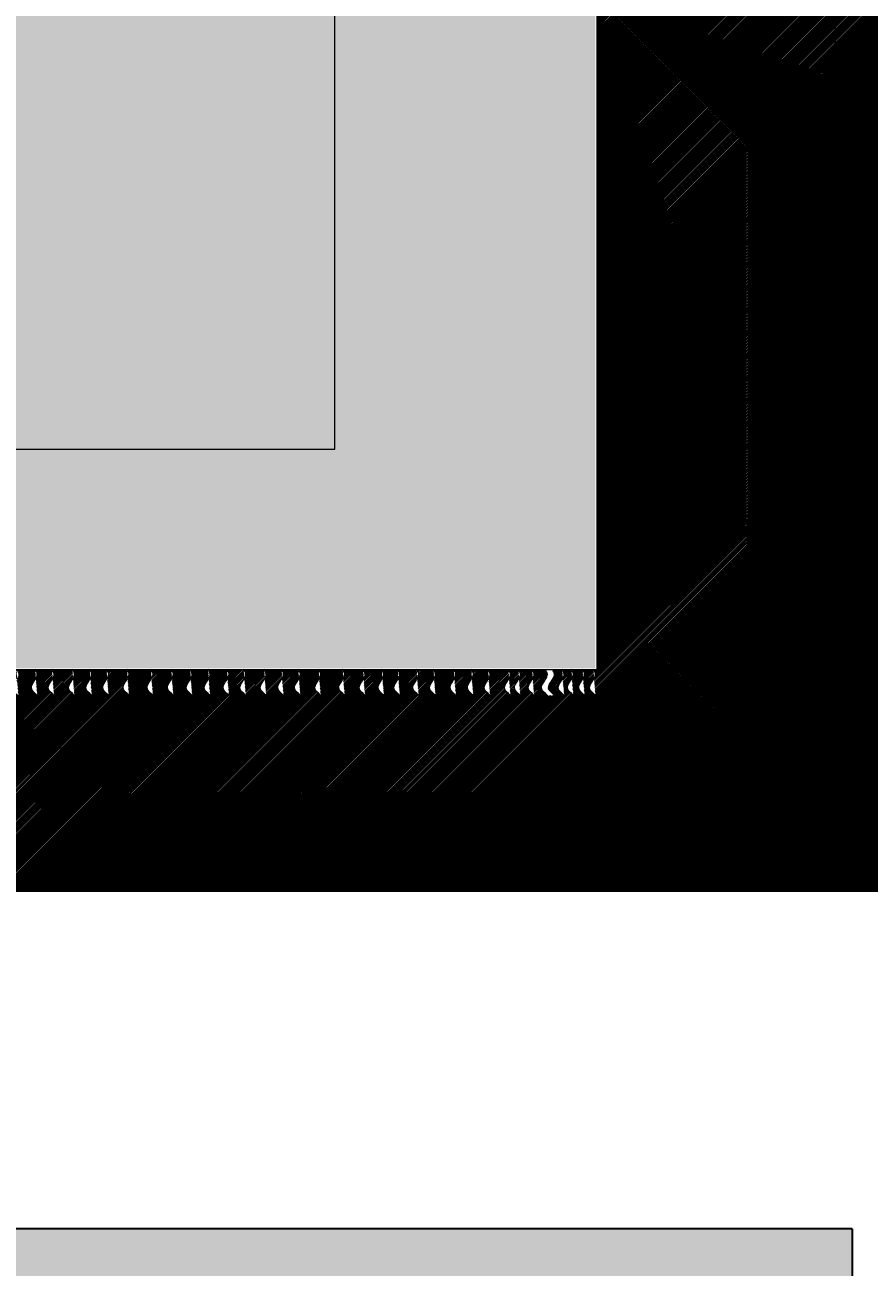
# Model space of a CAD drawing. Units: inches. Extents: x 192 to 1361, y -1362 to 367.
# Tile 5 of 23: x 396 to 495, y -761 to -616. Entities that reach past the tile are written whole.
import ezdxf

# ---------------------------------------------------------------- set-up
doc = ezdxf.new("R2010")
doc.units = ezdxf.units.IN
doc.header["$MEASUREMENT"] = 0
for name, color, linetype, lineweight in [('A-ANNO-DIMS', 2, 'Continuous', 18), ('A-FLOR', 8, 'Continuous', 18), ('A-WALL-PATT', 250, 'Continuous', 13), ('furniture', 32, 'Continuous', 18), ('walls', 7, 'Continuous', 35)]:
    doc.layers.add(name, color=color, linetype=linetype, lineweight=lineweight)
doc.layers.add('A-FLOR-PATT', color=254, linetype='Continuous', lineweight=13, true_color=0xfeeab9)
doc.layers.add('A-FURN-PATT', color=254, linetype='Continuous', lineweight=13, true_color=0xfeeab9)
doc.styles.get("Standard").update_dxf_attribs({"font": 'arial.ttf'})
doc.dimstyles.get("Standard").update_dxf_attribs({"dimtxt": 0.18, "dimasz": 0.18, "dimexe": 0.18, "dimexo": 0.0625, "dimgap": 0.09, "dimtad": 0, "dimtih": 1, "dimtoh": 1, "dimzin": 0, "dimdsep": 46, "dimlunit": 3, "dimtxsty": 'Standard', "dimcen": 0.09, "dimadec": 0, "dimazin": 0, "dimtfac": 1, "dimtofl": 0, "dimtmove": 0, "dimatfit": 3, "dimfxl": 1, "dimtolj": 1, "dimtzin": 0, "dimarcsym": 0})

# ---------------------------------------------------------------- blocks, each defined once
blk = doc.blocks.new('CARPET')
at = {"layer": 'furniture'}
for p, q in [((51.553, -55.124), (51.553, -98.109)), ((51.553, -98.109), (-51.535, -98.109))]:
    blk.add_line(p, q, dxfattribs=at)
for points, knots in [([(53.374, -58.593), (53.215, -58.395), (52.902, -58.005), (52.343, -58.395), (51.889, -58.678), (51.645, -58.504), (51.535, -58.426)], [0, 0, 0, 0, 0.653278, 1.290138, 1.740457, 2.114451, 2.114451, 2.114451, 2.114451]), ([(53.374, -59.78), (53.215, -59.582), (52.902, -59.192), (52.343, -59.582), (51.889, -59.864), (51.645, -59.691), (51.535, -59.612)], [0, 0, 0, 0, 0.653278, 1.290138, 1.740457, 2.114451, 2.114451, 2.114451, 2.114451]), ([(53.374, -61.218), (53.215, -61.02), (52.902, -60.63), (52.343, -61.02), (51.889, -61.302), (51.645, -61.129), (51.535, -61.051)], [0, 0, 0, 0, 0.653278, 1.290138, 1.740457, 2.114451, 2.114451, 2.114451, 2.114451]), ([(53.374, -62.444), (53.215, -62.247), (52.902, -61.857), (52.343, -62.247), (51.889, -62.529), (51.645, -62.355), (51.535, -62.277)], [0, 0, 0, 0, 0.653278, 1.290138, 1.740457, 2.114451, 2.114451, 2.114451, 2.114451]), ([(53.374, -63.631), (53.215, -63.433), (52.902, -63.043), (52.343, -63.433), (51.889, -63.715), (51.645, -63.542), (51.535, -63.463)], [0, 0, 0, 0, 0.653278, 1.290138, 1.740457, 2.114451, 2.114451, 2.114451, 2.114451]), ([(53.374, -65.069), (53.215, -64.872), (52.902, -64.481), (52.343, -64.871), (51.889, -65.154), (51.645, -64.98), (51.535, -64.902)], [0, 0, 0, 0, 0.653278, 1.290138, 1.740457, 2.114451, 2.114451, 2.114451, 2.114451]), ([(53.374, -66.759), (53.215, -66.561), (52.902, -66.171), (52.343, -66.561), (51.889, -66.844), (51.645, -66.67), (51.535, -66.592)], [0, 0, 0, 0, 0.653278, 1.290138, 1.740457, 2.114451, 2.114451, 2.114451, 2.114451]), ([(53.374, -68.197), (53.215, -68), (52.902, -67.61), (52.343, -68), (51.889, -68.282), (51.645, -68.109), (51.535, -68.03)], [0, 0, 0, 0, 0.653278, 1.290138, 1.740457, 2.114451, 2.114451, 2.114451, 2.114451]), ([(53.374, -69.528), (53.215, -69.33), (52.902, -68.94), (52.343, -69.33), (51.889, -69.612), (51.645, -69.439), (51.535, -69.36)], [0, 0, 0, 0, 0.653278, 1.290138, 1.740457, 2.114451, 2.114451, 2.114451, 2.114451]), ([(53.374, -70.794), (53.215, -70.596), (52.902, -70.206), (52.343, -70.596), (51.889, -70.878), (51.645, -70.705), (51.535, -70.626)], [0, 0, 0, 0, 0.653278, 1.290138, 1.740457, 2.114451, 2.114451, 2.114451, 2.114451]), ([(53.374, -72.124), (53.215, -71.927), (52.902, -71.536), (52.343, -71.927), (51.889, -72.209), (51.645, -72.035), (51.535, -71.957)], [0, 0, 0, 0, 0.653278, 1.290138, 1.740457, 2.114451, 2.114451, 2.114451, 2.114451]), ([(53.374, -73.311), (53.215, -73.113), (52.902, -72.723), (52.343, -73.113), (51.889, -73.395), (51.645, -73.222), (51.535, -73.143)], [0, 0, 0, 0, 0.653278, 1.290138, 1.740457, 2.114451, 2.114451, 2.114451, 2.114451]), ([(53.374, -74.749), (53.215, -74.551), (52.902, -74.161), (52.343, -74.551), (51.889, -74.833), (51.645, -74.66), (51.535, -74.582)], [0, 0, 0, 0, 0.653278, 1.290138, 1.740457, 2.114451, 2.114451, 2.114451, 2.114451]), ([(53.374, -75.975), (53.215, -75.778), (52.902, -75.388), (52.343, -75.778), (51.889, -76.06), (51.645, -75.887), (51.535, -75.808)], [0, 0, 0, 0, 0.653278, 1.290138, 1.740457, 2.114451, 2.114451, 2.114451, 2.114451]), ([(53.374, -77.162), (53.215, -76.964), (52.902, -76.574), (52.343, -76.964), (51.889, -77.246), (51.645, -77.073), (51.535, -76.995)], [0, 0, 0, 0, 0.653278, 1.290138, 1.740457, 2.114451, 2.114451, 2.114451, 2.114451]), ([(53.374, -78.6), (53.215, -78.403), (52.902, -78.012), (52.343, -78.403), (51.889, -78.685), (51.645, -78.511), (51.535, -78.433)], [0, 0, 0, 0, 0.653278, 1.290138, 1.740457, 2.114451, 2.114451, 2.114451, 2.114451]), ([(53.374, -80.29), (53.215, -80.093), (52.902, -79.702), (52.343, -80.093), (51.889, -80.375), (51.645, -80.201), (51.535, -80.123)], [0, 0, 0, 0, 0.653278, 1.290138, 1.740457, 2.114451, 2.114451, 2.114451, 2.114451]), ([(53.374, -81.728), (53.215, -81.531), (52.902, -81.141), (52.343, -81.531), (51.889, -81.813), (51.645, -81.64), (51.535, -81.561)], [0, 0, 0, 0, 0.653278, 1.290138, 1.740457, 2.114451, 2.114451, 2.114451, 2.114451]), ([(53.374, -83.059), (53.215, -82.861), (52.902, -82.471), (52.343, -82.861), (51.889, -83.143), (51.645, -82.97), (51.535, -82.891)], [0, 0, 0, 0, 0.653278, 1.290138, 1.740457, 2.114451, 2.114451, 2.114451, 2.114451]), ([(53.374, -84.183), (53.215, -83.985), (52.902, -83.595), (52.343, -83.985), (51.889, -84.267), (51.645, -84.094), (51.535, -84.015)], [0, 0, 0, 0, 0.653278, 1.290138, 1.740457, 2.114451, 2.114451, 2.114451, 2.114451]), ([(53.374, -85.513), (53.215, -85.316), (52.902, -84.926), (52.343, -85.316), (51.889, -85.598), (51.645, -85.424), (51.535, -85.346)], [0, 0, 0, 0, 0.653278, 1.290138, 1.740457, 2.114451, 2.114451, 2.114451, 2.114451]), ([(53.374, -86.7), (53.215, -86.502), (52.902, -86.112), (52.343, -86.502), (51.889, -86.784), (51.645, -86.611), (51.535, -86.532)], [0, 0, 0, 0, 0.653278, 1.290138, 1.740457, 2.114451, 2.114451, 2.114451, 2.114451]), ([(53.374, -88.138), (53.215, -87.941), (52.902, -87.55), (52.343, -87.94), (51.889, -88.223), (51.645, -88.049), (51.535, -87.971)], [0, 0, 0, 0, 0.653278, 1.290138, 1.740457, 2.114451, 2.114451, 2.114451, 2.114451]), ([(53.374, -89.364), (53.215, -89.167), (52.902, -88.777), (52.343, -89.167), (51.889, -89.449), (51.645, -89.276), (51.535, -89.197)], [0, 0, 0, 0, 0.653278, 1.290138, 1.740457, 2.114451, 2.114451, 2.114451, 2.114451]), ([(53.374, -90.551), (53.215, -90.353), (52.902, -89.963), (52.343, -90.353), (51.896, -90.633), (51.657, -90.468), (51.553, -90.396)], [0, 0, 0, 0, 0.653278, 1.290138, 1.740457, 2.0926, 2.0926, 2.0926, 2.0926]), ([(53.374, -91.989), (53.215, -91.792), (52.902, -91.402), (52.343, -91.791), (51.896, -92.071), (51.657, -91.907), (51.553, -91.835)], [0, 0, 0, 0, 0.653278, 1.290138, 1.740457, 2.0926, 2.0926, 2.0926, 2.0926]), ([(53.374, -92.689), (53.216, -92.489), (52.903, -92.093), (52.344, -92.492), (51.896, -92.771), (51.657, -92.607), (51.553, -92.535)], [0, 0, 0, 0, 0.656792, 1.295826, 1.746145, 2.098292, 2.098292, 2.098292, 2.098292]), ([(53.374, -93.659), (53.215, -93.462), (52.902, -93.072), (52.343, -93.461), (51.896, -93.741), (51.657, -93.577), (51.553, -93.505)], [0, 0, 0, 0, 0.653278, 1.290138, 1.740457, 2.0926, 2.0926, 2.0926, 2.0926]), ([(53.374, -94.594), (53.215, -94.396), (52.902, -94.006), (52.343, -94.395), (51.896, -94.676), (51.657, -94.511), (51.553, -94.439)], [0, 0, 0, 0, 0.653278, 1.290138, 1.740457, 2.0926, 2.0926, 2.0926, 2.0926]), ([(53.374, -95.098), (53.215, -94.9), (52.902, -94.51), (52.343, -94.899), (51.896, -95.179), (51.657, -95.015), (51.553, -94.943)], [0, 0, 0, 0, 0.653278, 1.290138, 1.740457, 2.0926, 2.0926, 2.0926, 2.0926]), ([(53.374, -95.78), (53.215, -95.583), (52.902, -95.193), (52.343, -95.583), (51.889, -95.865), (51.645, -95.692), (51.535, -95.613)], [0, 0, 0, 0, 0.653278, 1.290138, 1.740457, 2.114451, 2.114451, 2.114451, 2.114451]), ([(53.374, -96.428), (53.215, -96.23), (52.902, -95.84), (52.343, -96.23), (51.889, -96.512), (51.645, -96.339), (51.535, -96.261)], [0, 0, 0, 0, 0.653278, 1.290138, 1.740457, 2.114451, 2.114451, 2.114451, 2.114451]), ([(53.374, -97.219), (53.215, -97.021), (52.902, -96.631), (52.343, -97.021), (51.889, -97.303), (51.645, -97.13), (51.535, -97.051)], [0, 0, 0, 0, 0.653278, 1.290138, 1.740457, 2.114451, 2.114451, 2.114451, 2.114451]), ([(53.374, -97.991), (53.215, -97.793), (52.902, -97.403), (52.343, -97.793), (51.889, -98.075), (51.645, -97.902), (51.535, -97.824)], [0, 0, 0, 0, 0.653278, 1.290138, 1.740457, 2.114451, 2.114451, 2.114451, 2.114451])]:
    blk.add_open_spline(points, degree=3, knots=knots, dxfattribs=at)
blk = doc.blocks.new('A$C58D270C6')
at = {"layer": 'furniture'}
blk.add_lwpolyline([(0, 108), (77.905, 108), (77.905, 36), (0, 36)], close=True, dxfattribs=at)
at = {"layer": 'furniture', "xscale": 0.9312884925094044, "yscale": 0.9312884925094044, "zscale": 0.9312884925094044, "rotation": 90}
blk.add_blockref('CARPET', (3.79, 74.474), dxfattribs=at)
blk = doc.blocks.new('*D23')
at = {"layer": 'A-ANNO-DIMS', "color": 0, "lineweight": -2, "transparency": 16777216}
for p, q in [((463.14, -508.44), (491.09, -508.44)), ((490.91, -508.62), (490.91, -601.06)), ((490.91, -693.87), (490.91, -601.42)), ((463.14, -694.05), (491.09, -694.05))]:
    blk.add_line(p, q, dxfattribs=at)
at = {"layer": 'A-ANNO-DIMS', "color": 0, "transparency": 16777216}
for points in [[(490.88, -508.62), (490.94, -508.62), (490.91, -508.44)], [(490.88, -693.87), (490.94, -693.87), (490.91, -694.05)]]:
    blk.add_solid(points, dxfattribs=at)
at = {"layer": 'Defpoints', "color": 0, "transparency": 16777216}
for p in [(463.07, -508.44), (463.07, -694.05), (490.91, -694.05)]:
    blk.add_point(p, dxfattribs=at)
at = {"layer": 'A-ANNO-DIMS', "color": 0, "transparency": 16777216, "insert": (490.91, -601.24), "char_height": 0.18, "attachment_point": 5}
blk.add_mtext('\\A1;BED 186', dxfattribs=at)

msp = doc.modelspace()

# ---------------------------------------------------------------- hatches: boundary and pattern name
at = {"layer": 'A-FLOR-PATT'}
h = msp.add_hatch(dxfattribs=at)
h.set_pattern_fill('ANSI31', color=256)
edge = h.paths.add_edge_path()
edge.add_line((513.1511, -492.1899), (327.1032, -492.1899))
edge.add_line((327.1032, -492.1899), (327.1032, -508.439))
edge.add_line((327.1032, -508.439), (326.9465, -508.439))
edge.add_line((326.9465, -508.439), (326.6697, -537.1419))
edge.add_line((326.6697, -537.1419), (391.8439, -537.1419))
edge.add_line((391.8439, -537.1419), (391.8439, -520.2026))
edge.add_line((391.8439, -520.2026), (393.0084, -520.2026))
edge.add_spline(control_points=[(393.2858, -517.1545), (392.9584, -517.4172), (392.3119, -517.936), (392.9583, -518.8629), (393.4257, -519.6151), (393.1386, -520.0192), (393.0084, -520.2026)], knot_values=[0, 0, 0, 0, 0.65327829, 1.2901376, 1.74045698, 2.11445126, 2.11445126, 2.11445126, 2.11445126], degree=3, periodic=0)
edge.add_line((393.0084, -520.2026), (395.1098, -520.2026))
edge.add_spline(control_points=[(395.3872, -517.1545), (395.0598, -517.4172), (394.4133, -517.936), (395.0598, -518.8629), (395.5272, -519.6151), (395.2401, -520.0192), (395.1098, -520.2026)], knot_values=[0, 0, 0, 0, 0.65327829, 1.2901376, 1.74045698, 2.11445126, 2.11445126, 2.11445126, 2.11445126], degree=3, periodic=0)
edge.add_line((395.1098, -520.2026), (397.3144, -520.2026))
edge.add_spline(control_points=[(397.5918, -517.1545), (397.2644, -517.4172), (396.6179, -517.936), (397.2643, -518.8629), (397.7317, -519.6151), (397.4446, -520.0192), (397.3144, -520.2026)], knot_values=[0, 0, 0, 0, 0.65327829, 1.2901376, 1.74045698, 2.11445126, 2.11445126, 2.11445126, 2.11445126], degree=3, periodic=0)
edge.add_line((397.3144, -520.2026), (399.2806, -520.2026))
edge.add_spline(control_points=[(399.558, -517.1545), (399.2307, -517.4172), (398.5841, -517.936), (399.2306, -518.8629), (399.698, -519.6151), (399.4109, -520.0192), (399.2806, -520.2026)], knot_values=[0, 0, 0, 0, 0.65327829, 1.2901376, 1.74045698, 2.11445126, 2.11445126, 2.11445126, 2.11445126], degree=3, periodic=0)
edge.add_line((399.2806, -520.2026), (401.664, -520.2026))
edge.add_spline(control_points=[(401.9414, -517.1545), (401.614, -517.4172), (400.9675, -517.936), (401.6139, -518.8629), (402.0814, -519.6151), (401.7943, -520.0192), (401.664, -520.2026)], knot_values=[0, 0, 0, 0, 0.65327829, 1.2901376, 1.74045698, 2.11445126, 2.11445126, 2.11445126, 2.11445126], degree=3, periodic=0)
edge.add_line((401.664, -520.2026), (403.6961, -520.2026))
edge.add_spline(control_points=[(403.9735, -517.1545), (403.6461, -517.4172), (402.9996, -517.936), (403.6461, -518.8629), (404.1135, -519.6151), (403.8264, -520.0192), (403.6961, -520.2026)], knot_values=[0, 0, 0, 0, 0.65327829, 1.2901376, 1.74045698, 2.11445126, 2.11445126, 2.11445126, 2.11445126], degree=3, periodic=0)
edge.add_line((403.6961, -520.2026), (405.6624, -520.2026))
edge.add_spline(control_points=[(405.9398, -517.1545), (405.6124, -517.4172), (404.9659, -517.936), (405.6123, -518.8629), (406.0797, -519.6151), (405.7926, -520.0192), (405.6624, -520.2026)], knot_values=[0, 0, 0, 0, 0.65327829, 1.2901376, 1.74045698, 2.11445126, 2.11445126, 2.11445126, 2.11445126], degree=3, periodic=0)
edge.add_line((405.6624, -520.2026), (408.0457, -520.2026))
edge.add_spline(control_points=[(408.3231, -517.1545), (407.9958, -517.4172), (407.3493, -517.936), (407.9957, -518.8629), (408.4631, -519.6151), (408.176, -520.0192), (408.0457, -520.2026)], knot_values=[0, 0, 0, 0, 0.65327829, 1.2901376, 1.74045698, 2.11445126, 2.11445126, 2.11445126, 2.11445126], degree=3, periodic=0)
edge.add_line((408.0457, -520.2026), (410.8462, -520.2026))
edge.add_spline(control_points=[(411.1236, -517.1545), (410.7962, -517.4172), (410.1497, -517.936), (410.7961, -518.8629), (411.2635, -519.6151), (410.9764, -520.0192), (410.8462, -520.2026)], knot_values=[0, 0, 0, 0, 0.65327829, 1.2901376, 1.74045698, 2.11445126, 2.11445126, 2.11445126, 2.11445126], degree=3, periodic=0)
edge.add_line((410.8462, -520.2026), (413.2295, -520.2026))
edge.add_spline(control_points=[(413.5069, -517.1545), (413.1795, -517.4172), (412.533, -517.936), (413.1794, -518.8629), (413.6468, -519.6151), (413.3597, -520.0192), (413.2295, -520.2026)], knot_values=[0, 0, 0, 0, 0.65327829, 1.2901376, 1.74045698, 2.11445126, 2.11445126, 2.11445126, 2.11445126], degree=3, periodic=0)
edge.add_line((413.2295, -520.2026), (415.434, -520.2026))
edge.add_spline(control_points=[(415.7114, -517.1545), (415.3841, -517.4172), (414.7376, -517.936), (415.384, -518.8629), (415.8514, -519.6151), (415.5643, -520.0192), (415.434, -520.2026)], knot_values=[0, 0, 0, 0, 0.65327829, 1.2901376, 1.74045698, 2.11445126, 2.11445126, 2.11445126, 2.11445126], degree=3, periodic=0)
edge.add_line((415.434, -520.2026), (417.5321, -520.2026))
edge.add_spline(control_points=[(417.8095, -517.1545), (417.4821, -517.4172), (416.8356, -517.936), (417.482, -518.8629), (417.9494, -519.6151), (417.6623, -520.0192), (417.5321, -520.2026)], knot_values=[0, 0, 0, 0, 0.65327829, 1.2901376, 1.74045698, 2.11445126, 2.11445126, 2.11445126, 2.11445126], degree=3, periodic=0)
edge.add_line((417.5321, -520.2026), (419.7366, -520.2026))
edge.add_spline(control_points=[(420.014, -517.1545), (419.6867, -517.4172), (419.0401, -517.936), (419.6866, -518.8629), (420.154, -519.6151), (419.8669, -520.0192), (419.7366, -520.2026)], knot_values=[0, 0, 0, 0, 0.65327829, 1.2901376, 1.74045698, 2.11445126, 2.11445126, 2.11445126, 2.11445126], degree=3, periodic=0)
edge.add_line((419.7366, -520.2026), (421.7029, -520.2026))
edge.add_spline(control_points=[(421.9803, -517.1545), (421.6529, -517.4172), (421.0064, -517.936), (421.6528, -518.8629), (422.1202, -519.6151), (421.8331, -520.0192), (421.7029, -520.2026)], knot_values=[0, 0, 0, 0, 0.65327829, 1.2901376, 1.74045698, 2.11445126, 2.11445126, 2.11445126, 2.11445126], degree=3, periodic=0)
edge.add_line((421.7029, -520.2026), (424.0863, -520.2026))
edge.add_spline(control_points=[(424.3637, -517.1545), (424.0363, -517.4172), (423.3898, -517.936), (424.0362, -518.8629), (424.5036, -519.6151), (424.2165, -520.0192), (424.0863, -520.2026)], knot_values=[0, 0, 0, 0, 0.65327829, 1.2901376, 1.74045698, 2.11445126, 2.11445126, 2.11445126, 2.11445126], degree=3, periodic=0)
edge.add_line((424.0863, -520.2026), (426.1184, -520.2026))
edge.add_spline(control_points=[(426.3958, -517.1545), (426.0684, -517.4172), (425.4219, -517.936), (426.0683, -518.8629), (426.5357, -519.6151), (426.2486, -520.0192), (426.1184, -520.2026)], knot_values=[0, 0, 0, 0, 0.65327829, 1.2901376, 1.74045698, 2.11445126, 2.11445126, 2.11445126, 2.11445126], degree=3, periodic=0)
edge.add_line((426.1184, -520.2026), (428.0846, -520.2026))
edge.add_spline(control_points=[(428.362, -517.1545), (428.0346, -517.4172), (427.3881, -517.936), (428.0346, -518.8629), (428.502, -519.6151), (428.2149, -520.0192), (428.0846, -520.2026)], knot_values=[0, 0, 0, 0, 0.65327829, 1.2901376, 1.74045698, 2.11445126, 2.11445126, 2.11445126, 2.11445126], degree=3, periodic=0)
edge.add_line((428.0846, -520.2026), (430.468, -520.2026))
edge.add_spline(control_points=[(430.7454, -517.1545), (430.418, -517.4172), (429.7715, -517.936), (430.4179, -518.8629), (430.8853, -519.6151), (430.5983, -520.0192), (430.468, -520.2026)], knot_values=[0, 0, 0, 0, 0.65327829, 1.2901376, 1.74045698, 2.11445126, 2.11445126, 2.11445126, 2.11445126], degree=3, periodic=0)
edge.add_line((430.468, -520.2026), (433.2684, -520.2026))
edge.add_spline(control_points=[(433.5458, -517.1545), (433.2184, -517.4172), (432.5719, -517.936), (433.2184, -518.8629), (433.6858, -519.6151), (433.3987, -520.0192), (433.2684, -520.2026)], knot_values=[0, 0, 0, 0, 0.65327829, 1.2901376, 1.74045698, 2.11445126, 2.11445126, 2.11445126, 2.11445126], degree=3, periodic=0)
edge.add_line((433.2684, -520.2026), (435.6517, -520.2026))
edge.add_spline(control_points=[(435.9291, -517.1545), (435.6017, -517.4172), (434.9552, -517.936), (435.6017, -518.8629), (436.0691, -519.6151), (435.782, -520.0192), (435.6517, -520.2026)], knot_values=[0, 0, 0, 0, 0.65327829, 1.2901376, 1.74045698, 2.11445126, 2.11445126, 2.11445126, 2.11445126], degree=3, periodic=0)
edge.add_line((435.6517, -520.2026), (437.8563, -520.2026))
edge.add_spline(control_points=[(438.1337, -517.1545), (437.8063, -517.4172), (437.1598, -517.936), (437.8062, -518.8629), (438.2736, -519.6151), (437.9865, -520.0192), (437.8563, -520.2026)], knot_values=[0, 0, 0, 0, 0.65327829, 1.2901376, 1.74045698, 2.11445126, 2.11445126, 2.11445126, 2.11445126], degree=3, periodic=0)
edge.add_line((437.8563, -520.2026), (439.7189, -520.2026))
edge.add_spline(control_points=[(439.9963, -517.1545), (439.669, -517.4172), (439.0225, -517.936), (439.6689, -518.8629), (440.1363, -519.6151), (439.8492, -520.0192), (439.7189, -520.2026)], knot_values=[0, 0, 0, 0, 0.65327829, 1.2901376, 1.74045698, 2.11445126, 2.11445126, 2.11445126, 2.11445126], degree=3, periodic=0)
edge.add_line((439.7189, -520.2026), (441.9235, -520.2026))
edge.add_spline(control_points=[(442.2009, -517.1545), (441.8735, -517.4172), (441.227, -517.936), (441.8735, -518.8629), (442.3409, -519.6151), (442.0538, -520.0192), (441.9235, -520.2026)], knot_values=[0, 0, 0, 0, 0.65327829, 1.2901376, 1.74045698, 2.11445126, 2.11445126, 2.11445126, 2.11445126], degree=3, periodic=0)
edge.add_line((441.9235, -520.2026), (443.8898, -520.2026))
edge.add_spline(control_points=[(444.1672, -517.1545), (443.8398, -517.4172), (443.1933, -517.936), (443.8397, -518.8629), (444.3071, -519.6151), (444.02, -520.0192), (443.8898, -520.2026)], knot_values=[0, 0, 0, 0, 0.65327829, 1.2901376, 1.74045698, 2.11445126, 2.11445126, 2.11445126, 2.11445126], degree=3, periodic=0)
edge.add_line((443.8898, -520.2026), (446.2731, -520.2026))
edge.add_spline(control_points=[(446.5505, -517.1545), (446.2232, -517.4172), (445.5767, -517.936), (446.2231, -518.8629), (446.6905, -519.6151), (446.4034, -520.0192), (446.2731, -520.2026)], knot_values=[0, 0, 0, 0, 0.65327829, 1.2901376, 1.74045698, 2.11445126, 2.11445126, 2.11445126, 2.11445126], degree=3, periodic=0)
edge.add_line((446.2731, -520.2026), (448.3052, -520.2026))
edge.add_spline(control_points=[(448.5826, -517.1545), (448.2553, -517.4172), (447.6088, -517.936), (448.2552, -518.8629), (448.7226, -519.6151), (448.4355, -520.0192), (448.3052, -520.2026)], knot_values=[0, 0, 0, 0, 0.65327829, 1.2901376, 1.74045698, 2.11445126, 2.11445126, 2.11445126, 2.11445126], degree=3, periodic=0)
edge.add_line((448.3052, -520.2026), (450.2715, -520.2026))
edge.add_spline(control_points=[(450.5489, -517.1545), (450.2215, -517.4172), (449.575, -517.936), (450.2214, -518.8629), (450.6888, -519.6151), (450.4018, -520.0192), (450.2715, -520.2026)], knot_values=[0, 0, 0, 0, 0.65327829, 1.2901376, 1.74045698, 2.11445126, 2.11445126, 2.11445126, 2.11445126], degree=3, periodic=0)
edge.add_line((450.2715, -520.2026), (452.6549, -520.2026))
edge.add_spline(control_points=[(452.9323, -517.1545), (452.6049, -517.4172), (451.9584, -517.936), (452.6048, -518.8629), (453.0722, -519.6151), (452.7851, -520.0192), (452.6549, -520.2026)], knot_values=[0, 0, 0, 0, 0.65327829, 1.2901376, 1.74045698, 2.11445126, 2.11445126, 2.11445126, 2.11445126], degree=3, periodic=0)
edge.add_line((452.6549, -520.2026), (453.8151, -520.2026))
edge.add_spline(control_points=[(454.0925, -517.1545), (453.7499, -517.417), (453.0754, -517.9338), (453.769, -518.8576), (454.2314, -519.6154), (453.945, -520.0193), (453.8151, -520.2026)], knot_values=[0, 0, 0, 0, 0.6639037, 1.30740562, 1.757725, 2.13171928, 2.13171928, 2.13171928, 2.13171928], degree=3, periodic=0)
edge.add_line((453.8151, -520.2026), (455.3467, -520.2026))
edge.add_spline(control_points=[(455.6241, -517.1545), (455.2967, -517.4172), (454.6502, -517.936), (455.2967, -518.8629), (455.7641, -519.6151), (455.477, -520.0192), (455.3467, -520.2026)], knot_values=[0, 0, 0, 0, 0.65327829, 1.2901376, 1.74045698, 2.11445126, 2.11445126, 2.11445126, 2.11445126], degree=3, periodic=0)
edge.add_line((455.3467, -520.2026), (456.895, -520.2026))
edge.add_spline(control_points=[(456.895, -520.2026), (457.0253, -520.0192), (457.3124, -519.6151), (456.845, -518.8629), (456.1986, -517.936), (456.8451, -517.4172), (457.1724, -517.1545)], knot_values=[0, 0, 0, 0, 0.37399428, 0.82431366, 1.46117297, 2.11445126, 2.11445126, 2.11445126, 2.11445126], degree=3, periodic=0)
edge.add_spline(control_points=[(458.0074, -517.1545), (457.68, -517.4172), (457.0335, -517.936), (457.68, -518.8629), (458.1474, -519.6151), (457.8603, -520.0192), (457.73, -520.2026)], knot_values=[0, 0, 0, 0, 0.65327829, 1.2901376, 1.74045698, 2.11445126, 2.11445126, 2.11445126, 2.11445126], degree=3, periodic=0)
edge.add_line((457.73, -520.2026), (458.8613, -520.2026))
edge.add_spline(control_points=[(459.1387, -517.1545), (458.8113, -517.4172), (458.1648, -517.936), (458.8112, -518.8629), (459.2786, -519.6151), (458.9916, -520.0192), (458.8613, -520.2026)], knot_values=[0, 0, 0, 0, 0.65327829, 1.2901376, 1.74045698, 2.11445126, 2.11445126, 2.11445126, 2.11445126], degree=3, periodic=0)
edge.add_line((458.8613, -520.2026), (459.9346, -520.2026))
edge.add_spline(control_points=[(460.212, -517.1545), (459.8846, -517.4172), (459.2381, -517.936), (459.8845, -518.8629), (460.3519, -519.6151), (460.0648, -520.0192), (459.9346, -520.2026)], knot_values=[0, 0, 0, 0, 0.65327829, 1.2901376, 1.74045698, 2.11445126, 2.11445126, 2.11445126, 2.11445126], degree=3, periodic=0)
edge.add_line((459.9346, -520.2026), (461.2447, -520.2026))
edge.add_spline(control_points=[(461.5221, -517.1545), (461.1947, -517.4172), (460.5482, -517.936), (461.1946, -518.8629), (461.662, -519.6151), (461.3749, -520.0192), (461.2447, -520.2026)], knot_values=[0, 0, 0, 0, 0.65327829, 1.2901376, 1.74045698, 2.11445126, 2.11445126, 2.11445126, 2.11445126], degree=3, periodic=0)
edge.add_line((461.2447, -520.2026), (462.6002, -520.2026))
edge.add_spline(control_points=[(462.8776, -517.1545), (462.5502, -517.4172), (461.9037, -517.936), (462.5501, -518.8629), (463.0175, -519.6151), (462.7304, -520.0192), (462.6002, -520.2026)], knot_values=[0, 0, 0, 0, 0.65327829, 1.2901376, 1.74045698, 2.11445126, 2.11445126, 2.11445126, 2.11445126], degree=3, periodic=0)
edge.add_line((462.6002, -520.2026), (463.0739, -520.2026))
edge.add_line((463.0739, -520.2026), (463.0739, -691.0271))
edge.add_line((463.0739, -691.0271), (462.6214, -691.0271))
edge.add_spline(control_points=[(462.8776, -694.0453), (462.5502, -693.7826), (461.9037, -693.2638), (462.5501, -692.3369), (463.011, -691.5951), (462.7443, -691.2005), (462.6214, -691.0271)], knot_values=[0, 0, 0, 0, 0.65327829, 1.2901376, 1.74045698, 2.09412198, 2.09412198, 2.09412198, 2.09412198], degree=3, periodic=0)
edge.add_line((462.6214, -691.0271), (461.3416, -691.0271))
edge.add_spline(control_points=[(461.5978, -694.0453), (461.2704, -693.7826), (460.6239, -693.2638), (461.2703, -692.3369), (461.7312, -691.5951), (461.4644, -691.2005), (461.3416, -691.0271)], knot_values=[0, 0, 0, 0, 0.65327829, 1.2901376, 1.74045698, 2.09412198, 2.09412198, 2.09412198, 2.09412198], degree=3, periodic=0)
edge.add_line((461.3416, -691.0271), (460.0315, -691.0271))
edge.add_spline(control_points=[(460.2877, -694.0453), (459.9603, -693.7826), (459.3138, -693.2638), (459.9602, -692.3369), (460.4211, -691.5951), (460.1544, -691.2005), (460.0315, -691.0271)], knot_values=[0, 0, 0, 0, 0.65327829, 1.2901376, 1.74045698, 2.09412198, 2.09412198, 2.09412198, 2.09412198], degree=3, periodic=0)
edge.add_line((460.0315, -691.0271), (458.9582, -691.0271))
edge.add_spline(control_points=[(459.2144, -694.0453), (458.887, -693.7826), (458.2405, -693.2638), (458.8869, -692.3369), (459.3478, -691.5951), (459.0811, -691.2005), (458.9582, -691.0271)], knot_values=[0, 0, 0, 0, 0.65327829, 1.2901376, 1.74045698, 2.09412198, 2.09412198, 2.09412198, 2.09412198], degree=3, periodic=0)
edge.add_line((458.9582, -691.0271), (457.8269, -691.0271))
edge.add_spline(control_points=[(457.8269, -691.0271), (457.9464, -691.2008), (458.2187, -691.5966), (457.7545, -692.3366), (457.1096, -693.2638), (457.7558, -693.7826), (458.0831, -694.0453)], knot_values=[0, 0, 0, 0, 0.3521435, 0.80246288, 1.43932219, 2.09260048, 2.09260048, 2.09260048, 2.09260048], degree=3, periodic=0)
edge.add_spline(control_points=[(457.2481, -694.0453), (456.9209, -693.7826), (456.2746, -693.2638), (456.9195, -692.3366), (457.3837, -691.5966), (457.1114, -691.2008), (456.992, -691.0271)], knot_values=[0, 0, 0, 0, 0.65327829, 1.2901376, 1.74045698, 2.09260048, 2.09260048, 2.09260048, 2.09260048], degree=3, periodic=0)
edge.add_line((456.992, -691.0271), (455.4436, -691.0271))
edge.add_spline(control_points=[(455.6998, -694.0453), (455.3725, -693.7826), (454.7263, -693.2638), (455.3712, -692.3366), (455.8354, -691.5966), (455.5631, -691.2008), (455.4436, -691.0271)], knot_values=[0, 0, 0, 0, 0.65327829, 1.2901376, 1.74045698, 2.09260048, 2.09260048, 2.09260048, 2.09260048], degree=3, periodic=0)
edge.add_line((455.4436, -691.0271), (453.8363, -691.0271))
edge.add_spline(control_points=[(454.0925, -694.0453), (453.7602, -693.7827), (453.1046, -693.2646), (453.7653, -692.3383), (454.2277, -691.5965), (453.9557, -691.2008), (453.8363, -691.0271)], knot_values=[0, 0, 0, 0, 0.65679228, 1.29582582, 1.7461452, 2.0982924, 2.0982924, 2.0982924, 2.0982924], degree=3, periodic=0)
edge.add_line((453.8363, -691.0271), (452.6761, -691.0271))
edge.add_spline(control_points=[(452.9323, -694.0453), (452.605, -693.7826), (451.9587, -693.2638), (452.6037, -692.3366), (453.0678, -691.5966), (452.7956, -691.2008), (452.6761, -691.0271)], knot_values=[0, 0, 0, 0, 0.65327829, 1.2901376, 1.74045698, 2.09260048, 2.09260048, 2.09260048, 2.09260048], degree=3, periodic=0)
edge.add_line((452.6761, -691.0271), (450.2927, -691.0271))
edge.add_spline(control_points=[(450.5489, -694.0453), (450.2216, -693.7826), (449.5753, -693.2638), (450.2203, -692.3366), (450.6845, -691.5966), (450.4122, -691.2008), (450.2927, -691.0271)], knot_values=[0, 0, 0, 0, 0.65327829, 1.2901376, 1.74045698, 2.09260048, 2.09260048, 2.09260048, 2.09260048], degree=3, periodic=0)
edge.add_line((450.2927, -691.0271), (448.3265, -691.0271))
edge.add_spline(control_points=[(448.5826, -694.0453), (448.2553, -693.7826), (447.6088, -693.2638), (448.2552, -692.3369), (448.7161, -691.5951), (448.4493, -691.2005), (448.3265, -691.0271)], knot_values=[0, 0, 0, 0, 0.65327829, 1.2901376, 1.74045698, 2.09412198, 2.09412198, 2.09412198, 2.09412198], degree=3, periodic=0)
edge.add_line((448.3265, -691.0271), (446.2944, -691.0271))
edge.add_spline(control_points=[(446.5505, -694.0453), (446.2232, -693.7826), (445.5767, -693.2638), (446.2231, -692.3369), (446.684, -691.5951), (446.4172, -691.2005), (446.2944, -691.0271)], knot_values=[0, 0, 0, 0, 0.65327829, 1.2901376, 1.74045698, 2.09412198, 2.09412198, 2.09412198, 2.09412198], degree=3, periodic=0)
edge.add_line((446.2944, -691.0271), (443.911, -691.0271))
edge.add_spline(control_points=[(444.1672, -694.0453), (443.8398, -693.7826), (443.1933, -693.2638), (443.8397, -692.3369), (444.3006, -691.5951), (444.0338, -691.2005), (443.911, -691.0271)], knot_values=[0, 0, 0, 0, 0.65327829, 1.2901376, 1.74045698, 2.09412198, 2.09412198, 2.09412198, 2.09412198], degree=3, periodic=0)
edge.add_line((443.911, -691.0271), (441.9447, -691.0271))
edge.add_spline(control_points=[(442.2009, -694.0453), (441.8735, -693.7826), (441.227, -693.2638), (441.8735, -692.3369), (442.3344, -691.5951), (442.0676, -691.2005), (441.9447, -691.0271)], knot_values=[0, 0, 0, 0, 0.65327829, 1.2901376, 1.74045698, 2.09412198, 2.09412198, 2.09412198, 2.09412198], degree=3, periodic=0)
edge.add_line((441.9447, -691.0271), (439.7402, -691.0271))
edge.add_spline(control_points=[(439.9963, -694.0453), (439.669, -693.7826), (439.0225, -693.2638), (439.6689, -692.3369), (440.1298, -691.5951), (439.863, -691.2005), (439.7402, -691.0271)], knot_values=[0, 0, 0, 0, 0.65327829, 1.2901376, 1.74045698, 2.09412198, 2.09412198, 2.09412198, 2.09412198], degree=3, periodic=0)
edge.add_line((439.7402, -691.0271), (437.8775, -691.0271))
edge.add_spline(control_points=[(438.1337, -694.0453), (437.8063, -693.7826), (437.1598, -693.2638), (437.8062, -692.3369), (438.2671, -691.5951), (438.0004, -691.2005), (437.8775, -691.0271)], knot_values=[0, 0, 0, 0, 0.65327829, 1.2901376, 1.74045698, 2.09412198, 2.09412198, 2.09412198, 2.09412198], degree=3, periodic=0)
edge.add_line((437.8775, -691.0271), (435.6729, -691.0271))
edge.add_spline(control_points=[(435.9291, -694.0453), (435.6017, -693.7826), (434.9552, -693.2638), (435.6017, -692.3369), (436.0626, -691.5951), (435.7958, -691.2005), (435.6729, -691.0271)], knot_values=[0, 0, 0, 0, 0.65327829, 1.2901376, 1.74045698, 2.09412198, 2.09412198, 2.09412198, 2.09412198], degree=3, periodic=0)
edge.add_line((435.6729, -691.0271), (433.2896, -691.0271))
edge.add_spline(control_points=[(433.5458, -694.0453), (433.2184, -693.7826), (432.5719, -693.2638), (433.2184, -692.3369), (433.6793, -691.5951), (433.4125, -691.2005), (433.2896, -691.0271)], knot_values=[0, 0, 0, 0, 0.65327829, 1.2901376, 1.74045698, 2.09412198, 2.09412198, 2.09412198, 2.09412198], degree=3, periodic=0)
edge.add_line((433.2896, -691.0271), (430.4892, -691.0271))
edge.add_spline(control_points=[(430.7454, -694.0453), (430.418, -693.7826), (429.7715, -693.2638), (430.4179, -692.3369), (430.8788, -691.5951), (430.6121, -691.2005), (430.4892, -691.0271)], knot_values=[0, 0, 0, 0, 0.65327829, 1.2901376, 1.74045698, 2.09412198, 2.09412198, 2.09412198, 2.09412198], degree=3, periodic=0)
edge.add_line((430.4892, -691.0271), (428.1058, -691.0271))
edge.add_spline(control_points=[(428.362, -694.0453), (428.0346, -693.7826), (427.3881, -693.2638), (428.0346, -692.3369), (428.4955, -691.5951), (428.2287, -691.2005), (428.1058, -691.0271)], knot_values=[0, 0, 0, 0, 0.65327829, 1.2901376, 1.74045698, 2.09412198, 2.09412198, 2.09412198, 2.09412198], degree=3, periodic=0)
edge.add_line((428.1058, -691.0271), (426.1396, -691.0271))
edge.add_spline(control_points=[(426.3958, -694.0453), (426.0684, -693.7826), (425.4219, -693.2638), (426.0683, -692.3369), (426.5292, -691.5951), (426.2624, -691.2005), (426.1396, -691.0271)], knot_values=[0, 0, 0, 0, 0.65327829, 1.2901376, 1.74045698, 2.09412198, 2.09412198, 2.09412198, 2.09412198], degree=3, periodic=0)
edge.add_line((426.1396, -691.0271), (424.1075, -691.0271))
edge.add_spline(control_points=[(424.3637, -694.0453), (424.0363, -693.7826), (423.3898, -693.2638), (424.0362, -692.3369), (424.4971, -691.5951), (424.2303, -691.2005), (424.1075, -691.0271)], knot_values=[0, 0, 0, 0, 0.65327829, 1.2901376, 1.74045698, 2.09412198, 2.09412198, 2.09412198, 2.09412198], degree=3, periodic=0)
edge.add_line((424.1075, -691.0271), (421.7241, -691.0271))
edge.add_spline(control_points=[(421.9803, -694.0453), (421.6529, -693.7826), (421.0064, -693.2638), (421.6528, -692.3369), (422.1137, -691.5951), (421.847, -691.2005), (421.7241, -691.0271)], knot_values=[0, 0, 0, 0, 0.65327829, 1.2901376, 1.74045698, 2.09412198, 2.09412198, 2.09412198, 2.09412198], degree=3, periodic=0)
edge.add_line((421.7241, -691.0271), (419.7579, -691.0271))
edge.add_spline(control_points=[(420.014, -694.0453), (419.6867, -693.7826), (419.0401, -693.2638), (419.6866, -692.3369), (420.1475, -691.5951), (419.8807, -691.2005), (419.7579, -691.0271)], knot_values=[0, 0, 0, 0, 0.65327829, 1.2901376, 1.74045698, 2.09412198, 2.09412198, 2.09412198, 2.09412198], degree=3, periodic=0)
edge.add_line((419.7579, -691.0271), (417.5533, -691.0271))
edge.add_spline(control_points=[(417.8095, -694.0453), (417.4821, -693.7826), (416.8356, -693.2638), (417.482, -692.3369), (417.9429, -691.5951), (417.6761, -691.2005), (417.5533, -691.0271)], knot_values=[0, 0, 0, 0, 0.65327829, 1.2901376, 1.74045698, 2.09412198, 2.09412198, 2.09412198, 2.09412198], degree=3, periodic=0)
edge.add_line((417.5533, -691.0271), (415.4553, -691.0271))
edge.add_spline(control_points=[(415.7114, -694.0453), (415.3841, -693.7826), (414.7376, -693.2638), (415.384, -692.3369), (415.8449, -691.5951), (415.5781, -691.2005), (415.4553, -691.0271)], knot_values=[0, 0, 0, 0, 0.65327829, 1.2901376, 1.74045698, 2.09412198, 2.09412198, 2.09412198, 2.09412198], degree=3, periodic=0)
edge.add_line((415.4553, -691.0271), (413.2507, -691.0271))
edge.add_spline(control_points=[(413.5069, -694.0453), (413.1795, -693.7826), (412.533, -693.2638), (413.1794, -692.3369), (413.6403, -691.5951), (413.3736, -691.2005), (413.2507, -691.0271)], knot_values=[0, 0, 0, 0, 0.65327829, 1.2901376, 1.74045698, 2.09412198, 2.09412198, 2.09412198, 2.09412198], degree=3, periodic=0)
edge.add_line((413.2507, -691.0271), (410.8674, -691.0271))
edge.add_spline(control_points=[(411.1236, -694.0453), (410.7962, -693.7826), (410.1497, -693.2638), (410.7961, -692.3369), (411.257, -691.5951), (410.9903, -691.2005), (410.8674, -691.0271)], knot_values=[0, 0, 0, 0, 0.65327829, 1.2901376, 1.74045698, 2.09412198, 2.09412198, 2.09412198, 2.09412198], degree=3, periodic=0)
edge.add_line((410.8674, -691.0271), (408.067, -691.0271))
edge.add_spline(control_points=[(408.3231, -694.0453), (407.9958, -693.7826), (407.3493, -693.2638), (407.9957, -692.3369), (408.4566, -691.5951), (408.1898, -691.2005), (408.067, -691.0271)], knot_values=[0, 0, 0, 0, 0.65327829, 1.2901376, 1.74045698, 2.09412198, 2.09412198, 2.09412198, 2.09412198], degree=3, periodic=0)
edge.add_line((408.067, -691.0271), (405.6836, -691.0271))
edge.add_spline(control_points=[(405.9398, -694.0453), (405.6124, -693.7826), (404.9659, -693.2638), (405.6123, -692.3369), (406.0732, -691.5951), (405.8064, -691.2005), (405.6836, -691.0271)], knot_values=[0, 0, 0, 0, 0.65327829, 1.2901376, 1.74045698, 2.09412198, 2.09412198, 2.09412198, 2.09412198], degree=3, periodic=0)
edge.add_line((405.6836, -691.0271), (403.7173, -691.0271))
edge.add_spline(control_points=[(403.9735, -694.0453), (403.6461, -693.7826), (402.9996, -693.2638), (403.6461, -692.3369), (404.107, -691.5951), (403.8402, -691.2005), (403.7173, -691.0271)], knot_values=[0, 0, 0, 0, 0.65327829, 1.2901376, 1.74045698, 2.09412198, 2.09412198, 2.09412198, 2.09412198], degree=3, periodic=0)
edge.add_line((403.7173, -691.0271), (401.6852, -691.0271))
edge.add_spline(control_points=[(401.9414, -694.0453), (401.614, -693.7826), (400.9675, -693.2638), (401.6139, -692.3369), (402.0749, -691.5951), (401.8081, -691.2005), (401.6852, -691.0271)], knot_values=[0, 0, 0, 0, 0.65327829, 1.2901376, 1.74045698, 2.09412198, 2.09412198, 2.09412198, 2.09412198], degree=3, periodic=0)
edge.add_line((401.6852, -691.0271), (399.3019, -691.0271))
edge.add_spline(control_points=[(399.558, -694.0453), (399.2307, -693.7826), (398.5841, -693.2638), (399.2306, -692.3369), (399.6915, -691.5951), (399.4247, -691.2005), (399.3019, -691.0271)], knot_values=[0, 0, 0, 0, 0.65327829, 1.2901376, 1.74045698, 2.09412198, 2.09412198, 2.09412198, 2.09412198], degree=3, periodic=0)
edge.add_line((399.3019, -691.0271), (397.3356, -691.0271))
edge.add_spline(control_points=[(397.5918, -694.0453), (397.2644, -693.7826), (396.6179, -693.2638), (397.2643, -692.3369), (397.7252, -691.5951), (397.4585, -691.2005), (397.3356, -691.0271)], knot_values=[0, 0, 0, 0, 0.65327829, 1.2901376, 1.74045698, 2.09412198, 2.09412198, 2.09412198, 2.09412198], degree=3, periodic=0)
edge.add_line((397.3356, -691.0271), (395.131, -691.0271))
edge.add_spline(control_points=[(395.3872, -694.0453), (395.0598, -693.7826), (394.4133, -693.2638), (395.0598, -692.3369), (395.5207, -691.5951), (395.2539, -691.2005), (395.131, -691.0271)], knot_values=[0, 0, 0, 0, 0.65327829, 1.2901376, 1.74045698, 2.09412198, 2.09412198, 2.09412198, 2.09412198], degree=3, periodic=0)
edge.add_line((395.131, -691.0271), (393.0296, -691.0271))
edge.add_spline(control_points=[(393.2858, -694.0453), (392.9584, -693.7826), (392.3119, -693.2638), (392.9583, -692.3369), (393.4192, -691.5951), (393.1524, -691.2005), (393.0296, -691.0271)], knot_values=[0, 0, 0, 0, 0.65327829, 1.2901376, 1.74045698, 2.09412198, 2.09412198, 2.09412198, 2.09412198], degree=3, periodic=0)
edge.add_line((393.0296, -691.0271), (391.8439, -691.0271))
edge.add_line((391.8439, -691.0271), (391.8439, -665.2551))
edge.add_line((391.8439, -665.2551), (326.6697, -665.2551))
edge.add_line((326.6697, -665.2551), (326.3929, -693.958))
edge.add_line((326.3929, -693.958), (326.3929, -716.9381))
edge.add_line((326.3929, -716.9381), (513.1511, -716.9381))
edge.add_line((513.1511, -716.9381), (513.1511, -492.1899))
h.paths.add_polyline_path([(353.9763, -588.1534), (487.3258, -588.1534), (487.3258, -561.3965), (353.9763, -561.3965)], flags=25)
at = {"layer": 'A-FURN-PATT'}
h = msp.add_hatch(color=256, dxfattribs=at)
h.dxf.hatch_style = 1
h.paths.add_polyline_path([(320.1552, -604.3144), (300.7962, -604.3144), (300.7962, -641.8533), (320.1552, -641.8533)])
h.paths.add_polyline_path([(320.1552, -551.4593), (300.7962, -551.4593), (300.7962, -588.9983), (320.1552, -588.9983)])
h.paths.add_polyline_path([(462.8313, -520.0537), (391.6014, -520.0537), (391.6014, -536.993), (432.1311, -536.993), (432.1311, -665.1062), (391.6014, -665.1062), (391.6014, -690.8782), (462.8313, -690.8782)])
h = msp.add_hatch(color=256, dxfattribs=at)
h.dxf.hatch_style = 1
h.paths.add_polyline_path([(432.3737, -537.1419), (368.625, -537.1419), (368.625, -665.2551), (432.3737, -665.2551)])
h.paths.add_polyline_path([(368.625, -537.1419), (322.6088, -537.1419), (322.6088, -642.0022), (337.5553, -642.0022), (337.5553, -665.2551), (368.625, -665.2551)])
at = {"layer": 'A-WALL-PATT'}
h = msp.add_hatch(color=256, dxfattribs=at)
h.dxf.hatch_style = 1
h.paths.add_polyline_path([(309.5452, 191.102), (300.5452, 191.102), (300.5452, -126.898), (309.5452, -126.898), (309.5452, -117.898)])
h.paths.add_polyline_path([(420.798, 191.102), (337.3229, 191.102), (337.3229, 182.102), (420.798, 182.102)])
h.paths.add_polyline_path([(518.5452, 182.102), (625.4022, 182.102), (625.4022, 191.102), (509.5452, 191.102), (509.5452, 114.3262), (518.5452, 114.3262)])
h.paths.add_polyline_path([(842.5452, 191.102), (763.4438, 191.102), (763.4438, 182.102), (833.5452, 182.102), (833.5452, 161.1615), (836.8088, 161.1615), (842.5452, 161.1615)])
h.paths.add_polyline_path([(842.5452, -16.5675), (833.5452, -16.5675), (833.5452, -60.4996), (784.8041, -60.4996), (784.8041, -354.6796), (793.8041, -354.6796), (793.8041, -69.4996), (1094.1252, -69.4996), (1094.1252, -60.4996), (842.5452, -60.4996)])
h.paths.add_polyline_path([(518.5452, 36.602), (509.5452, 36.602), (509.5452, -117.898), (420.2204, -117.898), (420.2204, -126.898), (518.5452, -126.898)])
h.paths.add_polyline_path([(474.8041, -377.0384), (465.8041, -377.0384), (465.8041, -381.5384), (465.8041, -450.898), (537.5717, -450.898), (537.5717, -441.898), (474.8041, -441.898)])
h.paths.add_polyline_path([(1162.8041, -380.6763), (1204.3001, -380.6763), (1204.3001, -375.6763), (1195.1471, -375.6763), (1153.8041, -375.6763), (1153.8041, -448.4996), (856.5691, -448.4996), (856.5691, -457.4996), (1162.8041, -457.4996)])
h.paths.add_polyline_path([(1162.8041, -525.128), (1153.8041, -525.128), (1153.8041, -597.4996), (1162.8041, -597.4996)], flags=17)
h.paths.add_polyline_path([(1162.8041, -60.4996), (1153.8041, -60.4996), (1153.8041, -69.4996), (1153.8041, -177.4733), (1205.8889, -177.4733), (1205.8889, -172.4733), (1162.8041, -172.4733)])
h.paths.add_polyline_path([(980.5799, -525.686), (971.5799, -525.686), (971.5799, -597.4996), (980.5799, -597.4996)], flags=17)
h.paths.add_polyline_path([(856.5691, -448.4996), (798.7542, -448.4996), (784.8041, -448.4996), (784.8041, -457.4996), (847.5691, -457.4996), (847.5691, -597.4996), (784.8041, -597.4996), (784.8041, -606.4996), (1273.5658, -606.4996), (1273.5658, -597.4996), (856.5691, -597.4996)])
h.paths.add_polyline_path([(1273.5658, -773.892), (1099.8366, -773.892), (1099.8366, -851.9362), (1108.8366, -851.9362), (1108.8366, -782.892), (1273.5658, -782.892)])
h.paths.add_polyline_path([(1108.8366, -982.9214), (1099.8366, -982.9214), (1099.8366, -1067.6246), (1037.7563, -1067.6246), (1037.7563, -1076.6246), (1108.8366, -1076.6246)])
h.paths.add_polyline_path([(835.078, -1067.6246), (758.8458, -1067.6246), (758.8458, -940.2324), (749.8458, -940.2324), (749.8458, -963.172), (749.8458, -970.4644), (749.8458, -1076.6246), (835.078, -1076.6246)])
h.paths.add_polyline_path([(450.307, -1066.9838), (441.307, -1066.9838), (441.307, -1076.6246), (450.307, -1076.6246)])
h.paths.add_polyline_path([(492.8925, -756.4415), (274.8925, -756.4415), (274.8925, -765.4415), (492.8925, -765.4415)])
h.paths.add_polyline_path([(283.8925, -835.2244), (274.8925, -835.2244), (274.8925, -914.4415), (492.8925, -914.4415), (492.8925, -839.9415), (483.8925, -839.9415), (483.8925, -905.4415), (283.8925, -905.4415)])
h.paths.add_polyline_path([(283.8925, -441.898), (283.8925, -375.4296), (281.6021, -375.4296), (281.6021, -399.4121), (274.8925, -399.4121), (274.8925, -441.898), (274.8925, -684.5089), (283.8925, -684.5089)])

# ---------------------------------------------------------------- linework, layer by layer
at = {"layer": 'A-FLOR'}
msp.add_line((326.3929, -716.9381), (513.1511, -716.9381), dxfattribs=at)
at = {"layer": 'walls'}
for q in [(274.8925, -756.4415), (492.8925, -765.4415)]:
    msp.add_line((492.8925, -756.4415), q, dxfattribs=at)

# ---------------------------------------------------------------- block references
at = {"layer": 'furniture', "xscale": -1.779350280135438, "yscale": 1.779350280135438, "zscale": 1.779350280135438, "rotation": 180}
msp.add_blockref('A$C58D270C6', (293.7534, -473.0852), dxfattribs=at)

# ---------------------------------------------------------------- dimensions: what is measured, and where the dimension line sits
at = {"layer": 'A-ANNO-DIMS'}
dim = msp.add_linear_dim(base=(490.9148, -694.0453), p1=(463.0739, -508.439), p2=(463.0739, -694.0453), angle=270, text='BED <>', dimstyle='Standard', override={"dimdec": 0, "dimlfac": 1, "dimrnd": 0, "dimzin": 0, "dimdsep": 46, "dimlunit": 2}, dxfattribs=at)
dim.commit()
dim.dimension.update_dxf_attribs({"geometry": '*D23', "text_midpoint": (490.9148, -601.2421)})

doc.saveas('drawing.dxf')
